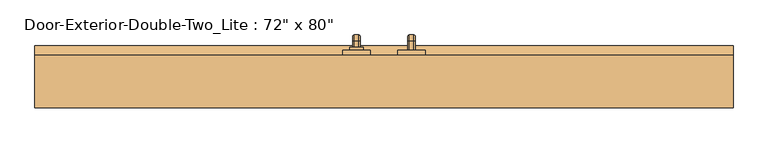
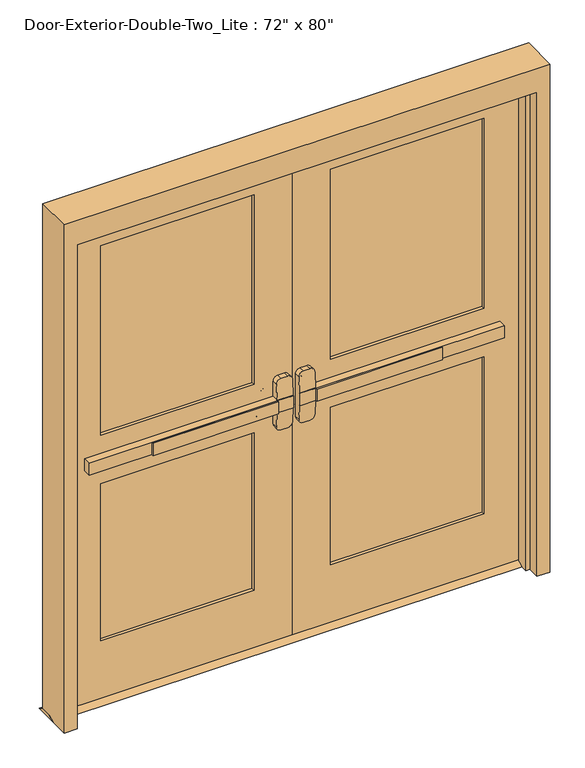
"""IFC4 building model written with IfcOpenShell, lengths in millimetres: door geometry."""

from ifc_helpers import new_model, si_unit, point, frame, frame_2d, origin, place, context, project, spatial, polyline, circle_curve, ellipse_curve, trimmed, segment, composite_curve, outline, extrude, faceted_brep, source, transform, mapped, element, save
from ifc_brep_helpers import plane_surface, cylinder_surface, revolved_surface, advanced_brep


def door_80c43283(model_context):
    return source(origin(), model_context, "Body", "SolidModel", [
        extrude(outline(polyline([(-575.7333333, 0.0), (-575.7333333, 6.35), (-76.2, 6.35), (-76.2, 0.0), (-575.7333333, 0.0)])), frame((0.0, 0.0, 990.6), z_axis=(0.0, 0.0, 1.0), x_axis=(1.0, 0.0, 0.0)), (0.0, 0.0, 1.0), 50.8),
        advanced_brep(
        [(-12.7, 6.35, 1041.4), (-76.2, 6.35, 1041.4), (-825.5, 6.35, 1041.4), (-825.5, 6.35, 990.6), (-76.2, 6.35, 990.6), (-12.7, 6.35, 990.6), (-825.5, 38.1, 1041.4), (-76.2, 38.1, 1041.4), (-76.2, 38.1, 1104.9), (-57.15, 38.1, 1123.95), (-31.75, 38.1, 1123.95), (-12.7, 38.1, 1104.9), (-12.7, 38.1, 927.1), (-31.75, 38.1, 908.05), (-57.15, 38.1, 908.05), (-76.2, 38.1, 927.1), (-76.2, 38.1, 990.6), (-825.5, 38.1, 990.6), (-12.7, 9.5252467, 1041.4), (-76.2, 9.5252467, 1041.4), (-12.7, 9.5252467, 990.6), (-12.7, 14.5354269, 927.1), (-12.7, 14.5354269, 1104.9), (-76.2, 9.5252467, 990.6), (-76.2, 14.5354269, 1104.9), (-76.2, 14.5354269, 927.1), (-57.15, 16.038481, 1123.95), (-31.75, 16.038481, 1123.95), (-31.75, 16.038481, 908.05), (-57.15, 16.038481, 908.05)],
        [
            (0, 1),
            (1, 2),
            (2, 3),
            (3, 4),
            (4, 5),
            (5, 0),
            (6, 7),
            (7, 8),
            (8, 9, circle_curve(frame((-57.15, 38.1, 1104.9), z_axis=(0.0, 1.0, 0.0), x_axis=(-1.0, 0.0, 0.0)), 19.05)),
            (9, 10),
            (10, 11, circle_curve(frame((-31.75, 38.1, 1104.9), z_axis=(0.0, 1.0, 0.0), x_axis=(-1.0, 0.0, 0.0)), 19.05)),
            (11, 12),
            (12, 13, circle_curve(frame((-31.75, 38.1, 927.1), z_axis=(0.0, 1.0, 0.0), x_axis=(-1.0, 0.0, 0.0)), 19.05)),
            (13, 14),
            (14, 15, circle_curve(frame((-57.15, 38.1, 927.1), z_axis=(0.0, 1.0, 0.0), x_axis=(-1.0, 0.0, 0.0)), 19.05)),
            (15, 16),
            (16, 17),
            (17, 6),
            (0, 18),
            (18, 19),
            (19, 7),
            (6, 2),
            (5, 20),
            (20, 21),
            (21, 12),
            (11, 22),
            (22, 18),
            (16, 23),
            (23, 20),
            (3, 17),
            (19, 24),
            (24, 8),
            (15, 25),
            (25, 23),
            (9, 26),
            (26, 27),
            (27, 10),
            (13, 28),
            (28, 29),
            (29, 14),
            (29, 25, ellipse_curve(frame((-57.15, 14.5354269, 927.1), z_axis=(0.0, 0.9969018152893365, 0.07865602756830282), x_axis=(0.0, -0.07865602756830208, 0.9969018152893365)), 19.1092038, 19.05)),
            (24, 26, ellipse_curve(frame((-57.15, 14.5354269, 1104.9), z_axis=(0.0, 0.9969018152893376, -0.07865602756828934), x_axis=(0.0, -0.078656027568288, -0.9969018152893377)), 19.1092038, 19.05)),
            (27, 22, ellipse_curve(frame((-31.75, 14.5354269, 1104.9), z_axis=(0.0, 0.9969018152893376, -0.07865602756828934), x_axis=(0.0, -0.078656027568288, -0.9969018152893377)), 19.1092038, 19.05)),
            (21, 28, ellipse_curve(frame((-31.75, 14.5354269, 927.1), z_axis=(0.0, 0.9969018152893365, 0.07865602756830282), x_axis=(0.0, -0.07865602756830208, 0.9969018152893365)), 19.1092038, 19.05)),
        ],
        [
            plane_surface(frame((-12.7, 6.35, 1041.4), z_axis=(0.0, -1.0, 0.0), x_axis=(1.0, 0.0, 0.0))),
            plane_surface(frame((-12.7, 38.1, 1041.4), z_axis=(0.0, 1.0, 0.0), x_axis=(-1.0, 0.0, 0.0))),
            plane_surface(frame((-825.5, 6.35, 1041.4), z_axis=(0.0, 0.0, 1.0), x_axis=(0.0, 1.0, 0.0))),
            plane_surface(frame((-12.7, 6.35, 1041.4), z_axis=(1.0, 0.0, 0.0), x_axis=(0.0, 1.0, 0.0))),
            plane_surface(frame((-12.7, 6.35, 990.6), z_axis=(0.0, 0.0, -1.0), x_axis=(0.0, 1.0, 0.0))),
            plane_surface(frame((-825.5, 6.35, 990.6), z_axis=(-1.0, 0.0, 0.0), x_axis=(0.0, 1.0, 0.0))),
            plane_surface(frame((-76.2, 9.5252467, 927.1), z_axis=(-1.0, 0.0, 0.0), x_axis=(0.0, 1.0, 0.0))),
            plane_surface(frame((-57.15, 9.5252467, 1123.95), z_axis=(0.0, 0.0, 1.0), x_axis=(0.0, 1.0, 0.0))),
            plane_surface(frame((-31.75, 9.5252467, 908.05), z_axis=(0.0, 0.0, -1.0), x_axis=(0.0, 1.0, 0.0))),
            cylinder_surface(frame((-57.15, 38.1, 927.1), z_axis=(0.0, -1.0, 0.0), x_axis=(-1.0, 0.0, 0.0)), 19.05),
            cylinder_surface(frame((-57.15, 38.1, 1104.9), z_axis=(0.0, -1.0, 0.0), x_axis=(-1.0, 0.0, 0.0)), 19.05),
            cylinder_surface(frame((-31.75, 38.1, 1104.9), z_axis=(0.0, -1.0, 0.0), x_axis=(-1.0, 0.0, 0.0)), 19.05),
            cylinder_surface(frame((-31.75, 38.1, 927.1), z_axis=(0.0, -1.0, 0.0), x_axis=(-1.0, 0.0, 0.0)), 19.05),
            plane_surface(frame((-76.2, 9.5252467, 1041.4), z_axis=(0.0, -0.9969018152893376, 0.07865602756828934), x_axis=(1.0, 0.0, 0.0))),
            plane_surface(frame((-76.2, 16.038481, 908.05), z_axis=(0.0, -0.9969018152893365, -0.07865602756830282), x_axis=(1.0, 0.0, 0.0))),
        ],
        [
            (0, [[1, 2, 3, 4, 5, 6]]),
            (1, [[7, 8, 9, 10, 11, 12, 13, 14, 15, 16, 17, 18]]),
            (2, [[-2, -1, 19, 20, 21, -7, 22]]),
            (3, [[23, 24, 25, -12, 26, 27, -19, -6]]),
            (4, [[-17, 28, 29, -23, -5, -4, 30]]),
            (5, [[-22, -18, -30, -3]]),
            (6, [[-21, 31, 32, -8]]),
            (6, [[33, 34, -28, -16]]),
            (7, [[35, 36, 37, -10]]),
            (8, [[38, 39, 40, -14]]),
            (9, [[-40, 41, -33, -15]]),
            (10, [[-32, 42, -35, -9]]),
            (11, [[-37, 43, -26, -11]]),
            (12, [[-25, 44, -38, -13]]),
            (13, [[-27, -43, -36, -42, -31, -20]]),
            (14, [[-29, -34, -41, -39, -44, -24]]),
        ],
    ),
        extrude(outline(polyline([(82.55, 12.7), (107.95, 0.0), (12.7, 0.0), (38.1, 12.7), (82.55, 12.7)])), frame((-965.2, 0.0, 0.0), z_axis=(1.0, 0.0, 0.0), x_axis=(0.0, 1.0, 0.0)), (0.0, 0.0, 1.0), 1930.4),
        extrude(outline(polyline([(575.7333333, 0.0), (76.2, 0.0), (76.2, 6.35), (575.7333333, 6.35), (575.7333333, 0.0)])), frame((0.0, 0.0, 990.6), z_axis=(0.0, 0.0, 1.0), x_axis=(1.0, 0.0, 0.0)), (0.0, 0.0, 1.0), 50.8),
        advanced_brep(
        [(12.7, 6.35, 1041.4), (12.7, 6.35, 990.6), (76.2, 6.35, 990.6), (825.5, 6.35, 990.6), (825.5, 6.35, 1041.4), (76.2, 6.35, 1041.4), (825.5, 38.1, 1041.4), (825.5, 38.1, 990.6), (76.2, 38.1, 990.6), (76.2, 38.1, 927.1), (57.15, 38.1, 908.05), (31.75, 38.1, 908.05), (12.7, 38.1, 927.1), (12.7, 38.1, 1104.9), (31.75, 38.1, 1123.95), (57.15, 38.1, 1123.95), (76.2, 38.1, 1104.9), (76.2, 38.1, 1041.4), (76.2, 9.5252467, 1041.4), (12.7, 9.5252467, 1041.4), (12.7, 14.5354269, 1104.9), (12.7, 14.5354269, 927.1), (12.7, 9.5252467, 990.6), (76.2, 9.5252467, 990.6), (76.2, 14.5354269, 927.1), (76.2, 14.5354269, 1104.9), (31.75, 16.038481, 1123.95), (57.15, 16.038481, 1123.95), (57.15, 16.038481, 908.05), (31.75, 16.038481, 908.05)],
        [
            (0, 1),
            (1, 2),
            (2, 3),
            (3, 4),
            (4, 5),
            (5, 0),
            (6, 7),
            (7, 8),
            (8, 9),
            (9, 10, circle_curve(frame((57.15, 38.1, 927.1), z_axis=(0.0, 1.0, 0.0), x_axis=(1.0, 0.0, 0.0)), 19.05)),
            (10, 11),
            (11, 12, circle_curve(frame((31.75, 38.1, 927.1), z_axis=(0.0, 1.0, 0.0), x_axis=(1.0, 0.0, 0.0)), 19.05)),
            (12, 13),
            (13, 14, circle_curve(frame((31.75, 38.1, 1104.9), z_axis=(0.0, 1.0, 0.0), x_axis=(1.0, 0.0, 0.0)), 19.05)),
            (14, 15),
            (15, 16, circle_curve(frame((57.15, 38.1, 1104.9), z_axis=(0.0, 1.0, 0.0), x_axis=(1.0, 0.0, 0.0)), 19.05)),
            (16, 17),
            (17, 6),
            (4, 6),
            (17, 18),
            (18, 19),
            (19, 0),
            (19, 20),
            (20, 13),
            (12, 21),
            (21, 22),
            (22, 1),
            (7, 3),
            (22, 23),
            (23, 8),
            (23, 24),
            (24, 9),
            (16, 25),
            (25, 18),
            (14, 26),
            (26, 27),
            (27, 15),
            (10, 28),
            (28, 29),
            (29, 11),
            (24, 28, ellipse_curve(frame((57.15, 14.5354269, 927.1), z_axis=(0.0, 0.9969018152893365, 0.07865602756830282), x_axis=(0.0, -0.07865602756830208, 0.9969018152893365)), 19.1092038, 19.05)),
            (27, 25, ellipse_curve(frame((57.15, 14.5354269, 1104.9), z_axis=(0.0, 0.9969018152893376, -0.07865602756828934), x_axis=(0.0, -0.078656027568288, -0.9969018152893377)), 19.1092038, 19.05)),
            (20, 26, ellipse_curve(frame((31.75, 14.5354269, 1104.9), z_axis=(0.0, 0.9969018152893376, -0.07865602756828934), x_axis=(0.0, -0.078656027568288, -0.9969018152893377)), 19.1092038, 19.05)),
            (29, 21, ellipse_curve(frame((31.75, 14.5354269, 927.1), z_axis=(0.0, 0.9969018152893365, 0.07865602756830282), x_axis=(0.0, -0.07865602756830208, 0.9969018152893365)), 19.1092038, 19.05)),
        ],
        [
            plane_surface(frame((12.7, 6.35, 1041.4), z_axis=(0.0, -1.0, 0.0), x_axis=(-1.0, 0.0, 0.0))),
            plane_surface(frame((12.7, 38.1, 1041.4), z_axis=(0.0, 1.0, 0.0), x_axis=(1.0, 0.0, 0.0))),
            plane_surface(frame((825.5, 6.35, 1041.4), z_axis=(0.0, 0.0, 1.0), x_axis=(0.0, 1.0, 0.0))),
            plane_surface(frame((12.7, 6.35, 1041.4), z_axis=(-1.0, 0.0, 0.0), x_axis=(0.0, 1.0, 0.0))),
            plane_surface(frame((12.7, 6.35, 990.6), z_axis=(0.0, 0.0, -1.0), x_axis=(0.0, 1.0, 0.0))),
            plane_surface(frame((825.5, 6.35, 990.6), z_axis=(1.0, 0.0, 0.0), x_axis=(0.0, 1.0, 0.0))),
            plane_surface(frame((76.2, 9.5252467, 927.1), z_axis=(1.0, 0.0, 0.0), x_axis=(0.0, 1.0, 0.0))),
            plane_surface(frame((57.15, 9.5252467, 1123.95), z_axis=(0.0, 0.0, 1.0), x_axis=(0.0, 1.0, 0.0))),
            plane_surface(frame((31.75, 9.5252467, 908.05), z_axis=(0.0, 0.0, -1.0), x_axis=(0.0, 1.0, 0.0))),
            cylinder_surface(frame((57.15, 38.1, 927.1), z_axis=(0.0, -1.0, 0.0), x_axis=(1.0, 0.0, 0.0)), 19.05),
            cylinder_surface(frame((57.15, 38.1, 1104.9), z_axis=(0.0, -1.0, 0.0), x_axis=(1.0, 0.0, 0.0)), 19.05),
            cylinder_surface(frame((31.75, 38.1, 1104.9), z_axis=(0.0, -1.0, 0.0), x_axis=(1.0, 0.0, 0.0)), 19.05),
            cylinder_surface(frame((31.75, 38.1, 927.1), z_axis=(0.0, -1.0, 0.0), x_axis=(1.0, 0.0, 0.0)), 19.05),
            plane_surface(frame((76.2, 9.5252467, 1041.4), z_axis=(0.0, -0.9969018152893376, 0.07865602756828934), x_axis=(-1.0, 0.0, 0.0))),
            plane_surface(frame((76.2, 16.038481, 908.05), z_axis=(0.0, -0.9969018152893365, -0.07865602756830282), x_axis=(-1.0, 0.0, 0.0))),
        ],
        [
            (0, [[1, 2, 3, 4, 5, 6]]),
            (1, [[7, 8, 9, 10, 11, 12, 13, 14, 15, 16, 17, 18]]),
            (2, [[19, -18, 20, 21, 22, -6, -5]]),
            (3, [[-1, -22, 23, 24, -13, 25, 26, 27]]),
            (4, [[28, -3, -2, -27, 29, 30, -8]]),
            (5, [[-4, -28, -7, -19]]),
            (6, [[-9, -30, 31, 32]]),
            (6, [[-17, 33, 34, -20]]),
            (7, [[-15, 35, 36, 37]]),
            (8, [[-11, 38, 39, 40]]),
            (9, [[-10, -32, 41, -38]]),
            (10, [[-16, -37, 42, -33]]),
            (11, [[-14, -24, 43, -35]]),
            (12, [[-12, -40, 44, -25]]),
            (13, [[-21, -34, -42, -36, -43, -23]]),
            (14, [[-26, -44, -39, -41, -31, -29]]),
        ],
    ),
        advanced_brep(
        [(66.2, 95.25, 1017.190625), (66.2, 95.25, 1014.809375), (69.771875, 95.25, 1011.2375), (82.6284594, 95.25, 1011.2375), (86.2, 95.25, 1014.8090406), (86.2, 95.25, 1017.190625), (82.628125, 95.25, 1020.7625), (69.771875, 95.25, 1020.7625), (66.2, 95.25, 887.809375), (69.771875, 95.25, 884.2375), (82.628125, 95.25, 884.2375), (86.2, 95.25, 887.809375), (86.2, 95.25, 890.1909594), (82.6284594, 95.25, 893.7625), (69.771875, 95.25, 893.7625), (66.2, 95.25, 890.190625), (66.2, 120.65, 1017.190625), (66.2, 134.540625, 1003.3), (66.2, 134.540625, 901.7), (66.2, 120.65, 887.809375), (66.2, 120.65, 890.190625), (66.2, 132.159375, 901.7), (66.2, 132.159375, 1003.3), (66.2, 120.65, 1014.809375), (69.771875, 120.65, 1011.2375), (82.6284594, 120.65, 1011.2375), (86.2, 120.65, 1014.8090406), (86.2, 132.1590406, 1003.3), (86.2, 132.1590406, 901.7), (86.2, 120.65, 890.1909594), (86.2, 120.65, 887.809375), (86.2, 134.540625, 901.7), (86.2, 134.540625, 1003.3), (86.2, 120.65, 1017.190625), (82.628125, 120.65, 1020.7625), (69.771875, 120.65, 1020.7625), (69.771875, 128.5875, 1003.3), (82.6284594, 128.5875, 1003.3), (82.628125, 138.1125, 1003.3), (69.771875, 138.1125, 1003.3), (69.771875, 128.5875, 901.7), (82.6284594, 128.5875, 901.7), (82.628125, 138.1125, 901.7), (69.771875, 138.1125, 901.7), (69.771875, 120.65, 893.7625), (82.6284594, 120.65, 893.7625), (82.628125, 120.65, 884.2375), (69.771875, 120.65, 884.2375)],
        [
            (0, 1),
            (1, 2, circle_curve(frame((69.771875, 95.25, 1014.809375), z_axis=(0.0, -1.0, 0.0), x_axis=(0.0, 0.0, 1.0)), 3.571875)),
            (2, 3),
            (3, 4, circle_curve(frame((82.6284594, 95.25, 1014.8090406), z_axis=(0.0, -1.0, 0.0), x_axis=(0.0, 0.0, 1.0)), 3.5715406)),
            (4, 5),
            (5, 6, circle_curve(frame((82.628125, 95.25, 1017.190625), z_axis=(0.0, -1.0, 0.0), x_axis=(0.0, 0.0, 1.0)), 3.571875)),
            (6, 7),
            (7, 0, circle_curve(frame((69.771875, 95.25, 1017.190625), z_axis=(0.0, -1.0, 0.0), x_axis=(0.0, 0.0, 1.0)), 3.571875)),
            (8, 9, circle_curve(frame((69.771875, 95.25, 887.809375), z_axis=(0.0, -1.0, 0.0), x_axis=(0.0, 0.0, -1.0)), 3.571875)),
            (9, 10),
            (10, 11, circle_curve(frame((82.628125, 95.25, 887.809375), z_axis=(0.0, -1.0, 0.0), x_axis=(0.0, 0.0, -1.0)), 3.571875)),
            (11, 12),
            (12, 13, circle_curve(frame((82.6284594, 95.25, 890.1909594), z_axis=(0.0, -1.0, 0.0), x_axis=(0.0, 0.0, -1.0)), 3.5715406)),
            (13, 14),
            (14, 15, circle_curve(frame((69.771875, 95.25, 890.190625), z_axis=(0.0, -1.0, 0.0), x_axis=(0.0, 0.0, -1.0)), 3.571875)),
            (15, 8),
            (0, 16),
            (16, 17, circle_curve(frame((66.2, 120.65, 1003.3), z_axis=(-1.0, 0.0, 0.0), x_axis=(0.0, 0.0, 1.0)), 13.890625)),
            (17, 18),
            (18, 19, circle_curve(frame((66.2, 120.65, 901.7), z_axis=(-1.0, 0.0, 0.0), x_axis=(0.0, 1.0, 0.0)), 13.890625)),
            (19, 8),
            (15, 20),
            (20, 21, circle_curve(frame((66.2, 120.65, 901.7), z_axis=(1.0, 0.0, 0.0), x_axis=(0.0, 1.0, 0.0)), 11.509375)),
            (21, 22),
            (22, 23, circle_curve(frame((66.2, 120.65, 1003.3), z_axis=(1.0, 0.0, 0.0), x_axis=(0.0, 0.0, 1.0)), 11.509375)),
            (23, 1),
            (23, 24, circle_curve(frame((69.771875, 120.65, 1014.809375), z_axis=(0.0, -1.0, 0.0), x_axis=(0.0, 0.0, 1.0)), 3.571875)),
            (24, 2),
            (24, 25),
            (25, 3),
            (25, 26, circle_curve(frame((82.6284594, 120.65, 1014.8090406), z_axis=(0.0, -1.0, 0.0), x_axis=(0.0, 0.0, 1.0)), 3.5715406)),
            (26, 4),
            (26, 27, circle_curve(frame((86.2, 120.65, 1003.3), z_axis=(-1.0, 0.0, 0.0), x_axis=(0.0, 0.0, 1.0)), 11.5090406)),
            (27, 28),
            (28, 29, circle_curve(frame((86.2, 120.65, 901.7), z_axis=(-1.0, 0.0, 0.0), x_axis=(0.0, 1.0, 0.0)), 11.5090406)),
            (29, 12),
            (11, 30),
            (30, 31, circle_curve(frame((86.2, 120.65, 901.7), z_axis=(1.0, 0.0, 0.0), x_axis=(0.0, 1.0, 0.0)), 13.890625)),
            (31, 32),
            (32, 33, circle_curve(frame((86.2, 120.65, 1003.3), z_axis=(1.0, 0.0, 0.0), x_axis=(0.0, 0.0, 1.0)), 13.890625)),
            (33, 5),
            (33, 34, circle_curve(frame((82.628125, 120.65, 1017.190625), z_axis=(0.0, -1.0, 0.0), x_axis=(0.0, 0.0, 1.0)), 3.571875)),
            (34, 6),
            (34, 35),
            (35, 7),
            (35, 16, circle_curve(frame((69.771875, 120.65, 1017.190625), z_axis=(0.0, -1.0, 0.0), x_axis=(0.0, 0.0, 1.0)), 3.571875)),
            (36, 24, circle_curve(frame((69.771875, 120.65, 1003.3), z_axis=(1.0, 0.0, 0.0), x_axis=(0.0, 0.0, 1.0)), 7.9375)),
            (22, 36, circle_curve(frame((69.771875, 132.159375, 1003.3), z_axis=(0.0, 0.0, 1.0), x_axis=(0.0, 1.0, 0.0)), 3.571875)),
            (37, 25, circle_curve(frame((82.6284594, 120.65, 1003.3), z_axis=(1.0, 0.0, 0.0), x_axis=(0.0, 0.0, 1.0)), 7.9375)),
            (36, 37),
            (37, 27, circle_curve(frame((82.6284594, 132.1590406, 1003.3), z_axis=(0.0, 0.0, 1.0), x_axis=(0.0, 1.0, 0.0)), 3.5715406)),
            (38, 34, circle_curve(frame((82.628125, 120.65, 1003.3), z_axis=(1.0, 0.0, 0.0), x_axis=(0.0, 0.0, 1.0)), 17.4625)),
            (32, 38, circle_curve(frame((82.628125, 134.540625, 1003.3), z_axis=(0.0, 0.0, 1.0), x_axis=(0.0, 1.0, 0.0)), 3.571875)),
            (39, 35, circle_curve(frame((69.771875, 120.65, 1003.3), z_axis=(1.0, 0.0, 0.0), x_axis=(0.0, 0.0, 1.0)), 17.4625)),
            (38, 39),
            (39, 17, circle_curve(frame((69.771875, 134.540625, 1003.3), z_axis=(0.0, 0.0, 1.0), x_axis=(0.0, 1.0, 0.0)), 3.571875)),
            (21, 40, circle_curve(frame((69.771875, 132.159375, 901.7), z_axis=(0.0, 0.0, 1.0), x_axis=(0.0, 1.0, 0.0)), 3.571875)),
            (40, 36),
            (40, 41),
            (41, 37),
            (41, 28, circle_curve(frame((82.6284594, 132.1590406, 901.7), z_axis=(0.0, 0.0, 1.0), x_axis=(0.0, 1.0, 0.0)), 3.5715406)),
            (31, 42, circle_curve(frame((82.628125, 134.540625, 901.7), z_axis=(0.0, 0.0, 1.0), x_axis=(0.0, 1.0, 0.0)), 3.571875)),
            (42, 38),
            (42, 43),
            (43, 39),
            (43, 18, circle_curve(frame((69.771875, 134.540625, 901.7), z_axis=(0.0, 0.0, 1.0), x_axis=(0.0, 1.0, 0.0)), 3.571875)),
            (44, 40, circle_curve(frame((69.771875, 120.65, 901.7), z_axis=(1.0, 0.0, 0.0), x_axis=(0.0, 1.0, 0.0)), 7.9375)),
            (20, 44, circle_curve(frame((69.771875, 120.65, 890.190625), z_axis=(0.0, 1.0, 0.0), x_axis=(0.0, 0.0, -1.0)), 3.571875)),
            (45, 41, circle_curve(frame((82.6284594, 120.65, 901.7), z_axis=(1.0, 0.0, 0.0), x_axis=(0.0, 1.0, 0.0)), 7.9375)),
            (44, 45),
            (45, 29, circle_curve(frame((82.6284594, 120.65, 890.1909594), z_axis=(0.0, 1.0, 0.0), x_axis=(0.0, 0.0, -1.0)), 3.5715406)),
            (46, 42, circle_curve(frame((82.628125, 120.65, 901.7), z_axis=(1.0, 0.0, 0.0), x_axis=(0.0, 1.0, 0.0)), 17.4625)),
            (30, 46, circle_curve(frame((82.628125, 120.65, 887.809375), z_axis=(0.0, 1.0, 0.0), x_axis=(0.0, 0.0, -1.0)), 3.571875)),
            (47, 43, circle_curve(frame((69.771875, 120.65, 901.7), z_axis=(1.0, 0.0, 0.0), x_axis=(0.0, 1.0, 0.0)), 17.4625)),
            (46, 47),
            (47, 19, circle_curve(frame((69.771875, 120.65, 887.809375), z_axis=(0.0, 1.0, 0.0), x_axis=(0.0, 0.0, -1.0)), 3.571875)),
            (14, 44),
            (13, 45),
            (10, 46),
            (9, 47),
        ],
        [
            plane_surface(frame((76.2, 95.25, 1016.0), z_axis=(0.0, -1.0, 0.0), x_axis=(1.0, 0.0, 0.0))),
            plane_surface(frame((76.2, 95.25, 889.0), z_axis=(0.0, -1.0, 0.0), x_axis=(1.0, 0.0, 0.0))),
            plane_surface(frame((66.2, 95.25, 1017.190625), z_axis=(-1.0, 0.0, 0.0), x_axis=(0.0, 1.0, 0.0))),
            cylinder_surface(frame((69.771875, 95.25, 1014.809375), z_axis=(0.0, -1.0, 0.0), x_axis=(0.0, 0.0, 1.0)), 3.571875),
            plane_surface(frame((69.771875, 95.25, 1011.2375), z_axis=(0.0, 0.0, -1.0), x_axis=(0.0, 1.0, 0.0))),
            cylinder_surface(frame((82.6284594, 95.25, 1014.8090406), z_axis=(0.0, -1.0, 0.0), x_axis=(0.0, 0.0, 1.0)), 3.5715406),
            plane_surface(frame((86.2, 95.25, 1014.8090406), z_axis=(1.0, 0.0, 0.0), x_axis=(0.0, 1.0, 0.0))),
            cylinder_surface(frame((82.628125, 95.25, 1017.190625), z_axis=(0.0, -1.0, 0.0), x_axis=(0.0, 0.0, 1.0)), 3.571875),
            plane_surface(frame((82.628125, 95.25, 1020.7625), z_axis=(0.0, 0.0, 1.0), x_axis=(0.0, 1.0, 0.0))),
            cylinder_surface(frame((69.771875, 95.25, 1017.190625), z_axis=(0.0, -1.0, 0.0), x_axis=(0.0, 0.0, 1.0)), 3.571875),
            revolved_surface(trimmed(ellipse_curve(frame((69.771875, 120.65, 1014.809375), z_axis=(0.0, -1.0, 0.0), x_axis=(0.0, 0.0, 1.0)), 3.571875, 3.571875), [point((66.2, 120.65, 1014.809375))], [point((69.771875, 120.65, 1011.2375))], True, "CARTESIAN"), (76.2, 120.65, 1003.3), (-1.0, 0.0, 0.0)),
            revolved_surface(polyline([(69.771875, 120.65, 1011.2375), (82.6284594, 120.65, 1011.2375)]), (76.2, 120.65, 1003.3), (-1.0, 0.0, 0.0)),
            revolved_surface(trimmed(ellipse_curve(frame((82.6284594, 120.65, 1014.8090406), z_axis=(0.0, -1.0, 0.0), x_axis=(0.0, 0.0, 1.0)), 3.5715406, 3.5715406), [point((82.6284594, 120.65, 1011.2375))], [point((86.2, 120.65, 1014.8090406))], True, "CARTESIAN"), (76.2, 120.65, 1003.3), (-1.0, 0.0, 0.0)),
            revolved_surface(trimmed(ellipse_curve(frame((82.628125, 120.65, 1017.190625), z_axis=(0.0, -1.0, 0.0), x_axis=(0.0, 0.0, 1.0)), 3.571875, 3.571875), [point((86.2, 120.65, 1017.190625))], [point((82.628125, 120.65, 1020.7625))], True, "CARTESIAN"), (76.2, 120.65, 1003.3), (-1.0, 0.0, 0.0)),
            cylinder_surface(frame((76.2, 120.65, 1003.3), z_axis=(-1.0, 0.0, 0.0), x_axis=(0.0, 0.0, 1.0)), 17.4625),
            revolved_surface(trimmed(ellipse_curve(frame((69.771875, 120.65, 1017.190625), z_axis=(0.0, -1.0, 0.0), x_axis=(0.0, 0.0, 1.0)), 3.571875, 3.571875), [point((69.771875, 120.65, 1020.7625))], [point((66.2, 120.65, 1017.190625))], True, "CARTESIAN"), (76.2, 120.65, 1003.3), (-1.0, 0.0, 0.0)),
            cylinder_surface(frame((69.771875, 132.159375, 1003.3), z_axis=(0.0, 0.0, 1.0), x_axis=(0.0, 1.0, 0.0)), 3.571875),
            plane_surface(frame((69.771875, 128.5875, 1003.3), z_axis=(0.0, -1.0, 0.0), x_axis=(0.0, 0.0, -1.0))),
            cylinder_surface(frame((82.6284594, 132.1590406, 1003.3), z_axis=(0.0, 0.0, 1.0), x_axis=(0.0, 1.0, 0.0)), 3.5715406),
            cylinder_surface(frame((82.628125, 134.540625, 1003.3), z_axis=(0.0, 0.0, 1.0), x_axis=(0.0, 1.0, 0.0)), 3.571875),
            plane_surface(frame((82.628125, 138.1125, 1003.3), z_axis=(0.0, 1.0, 0.0), x_axis=(0.0, 0.0, -1.0))),
            cylinder_surface(frame((69.771875, 134.540625, 1003.3), z_axis=(0.0, 0.0, 1.0), x_axis=(0.0, 1.0, 0.0)), 3.571875),
            revolved_surface(trimmed(ellipse_curve(frame((69.771875, 132.159375, 901.7), z_axis=(0.0, 0.0, 1.0), x_axis=(0.0, 1.0, 0.0)), 3.571875, 3.571875), [point((66.2, 132.159375, 901.7))], [point((69.771875, 128.5875, 901.7))], True, "CARTESIAN"), (76.2, 120.65, 901.7), (-1.0, 0.0, 0.0)),
            revolved_surface(polyline([(69.771875, 128.5875, 901.7), (82.6284594, 128.5875, 901.7)]), (76.2, 120.65, 901.7), (-1.0, 0.0, 0.0)),
            revolved_surface(trimmed(ellipse_curve(frame((82.6284594, 132.1590406, 901.7), z_axis=(0.0, 0.0, 1.0), x_axis=(0.0, 1.0, 0.0)), 3.5715406, 3.5715406), [point((82.6284594, 128.5875, 901.7))], [point((86.2, 132.1590406, 901.7))], True, "CARTESIAN"), (76.2, 120.65, 901.7), (-1.0, 0.0, 0.0)),
            revolved_surface(trimmed(ellipse_curve(frame((82.628125, 134.540625, 901.7), z_axis=(0.0, 0.0, 1.0), x_axis=(0.0, 1.0, 0.0)), 3.571875, 3.571875), [point((86.2, 134.540625, 901.7))], [point((82.628125, 138.1125, 901.7))], True, "CARTESIAN"), (76.2, 120.65, 901.7), (-1.0, 0.0, 0.0)),
            cylinder_surface(frame((76.2, 120.65, 901.7), z_axis=(-1.0, 0.0, 0.0), x_axis=(0.0, 1.0, 0.0)), 17.4625),
            revolved_surface(trimmed(ellipse_curve(frame((69.771875, 134.540625, 901.7), z_axis=(0.0, 0.0, 1.0), x_axis=(0.0, 1.0, 0.0)), 3.571875, 3.571875), [point((69.771875, 138.1125, 901.7))], [point((66.2, 134.540625, 901.7))], True, "CARTESIAN"), (76.2, 120.65, 901.7), (-1.0, 0.0, 0.0)),
            cylinder_surface(frame((69.771875, 120.65, 890.190625), z_axis=(0.0, 1.0, 0.0), x_axis=(0.0, 0.0, -1.0)), 3.571875),
            plane_surface(frame((69.771875, 120.65, 893.7625), z_axis=(0.0, 0.0, 1.0), x_axis=(0.0, -1.0, 0.0))),
            cylinder_surface(frame((82.6284594, 120.65, 890.1909594), z_axis=(0.0, 1.0, 0.0), x_axis=(0.0, 0.0, -1.0)), 3.5715406),
            cylinder_surface(frame((82.628125, 120.65, 887.809375), z_axis=(0.0, 1.0, 0.0), x_axis=(0.0, 0.0, -1.0)), 3.571875),
            plane_surface(frame((82.628125, 120.65, 884.2375), z_axis=(0.0, 0.0, -1.0), x_axis=(0.0, -1.0, 0.0))),
            cylinder_surface(frame((69.771875, 120.65, 887.809375), z_axis=(0.0, 1.0, 0.0), x_axis=(0.0, 0.0, -1.0)), 3.571875),
        ],
        [
            (0, [[1, 2, 3, 4, 5, 6, 7, 8]]),
            (1, [[9, 10, 11, 12, 13, 14, 15, 16]]),
            (2, [[-1, 17, 18, 19, 20, 21, -16, 22, 23, 24, 25, 26]]),
            (3, [[-2, -26, 27, 28]]),
            (4, [[-3, -28, 29, 30]]),
            (5, [[-4, -30, 31, 32]]),
            (6, [[-5, -32, 33, 34, 35, 36, -12, 37, 38, 39, 40, 41]]),
            (7, [[-6, -41, 42, 43]]),
            (8, [[-7, -43, 44, 45]]),
            (9, [[-8, -45, 46, -17]]),
            (10, [[47, -27, -25, 48]]),
            (11, [[49, -29, -47, 50]]),
            (12, [[-33, -31, -49, 51]]),
            (13, [[52, -42, -40, 53]]),
            (14, [[54, -44, -52, 55]]),
            (15, [[-18, -46, -54, 56]]),
            (16, [[-48, -24, 57, 58]]),
            (17, [[-50, -58, 59, 60]]),
            (18, [[-51, -60, 61, -34]]),
            (19, [[-53, -39, 62, 63]]),
            (20, [[-55, -63, 64, 65]]),
            (21, [[-56, -65, 66, -19]]),
            (22, [[67, -57, -23, 68]]),
            (23, [[69, -59, -67, 70]]),
            (24, [[-35, -61, -69, 71]]),
            (25, [[72, -62, -38, 73]]),
            (26, [[74, -64, -72, 75]]),
            (27, [[-20, -66, -74, 76]]),
            (28, [[-68, -22, -15, 77]]),
            (29, [[-70, -77, -14, 78]]),
            (30, [[-71, -78, -13, -36]]),
            (31, [[-73, -37, -11, 79]]),
            (32, [[-75, -79, -10, 80]]),
            (33, [[-76, -80, -9, -21]]),
        ],
    ),
        extrude(outline(composite_curve([segment(trimmed(circle_curve(frame_2d((1113.0338574, 76.2)), 89.3016225), [point((1193.8, 114.3))], [point((1193.8, 38.1))], False, "CARTESIAN"), True, "CONTINUOUS"), segment(polyline([(1193.8, 38.1), (838.2, 38.1)]), True, "CONTINUOUS"), segment(trimmed(circle_curve(frame_2d((918.9661426, 76.2)), 89.3016225), [point((838.2, 38.1))], [point((838.2, 114.3))], False, "CARTESIAN"), True, "CONTINUOUS"), segment(polyline([(838.2, 114.3), (1193.8, 114.3)]), True, "CONTINUOUS")], self_intersect=False)), frame((0.0, 82.55, 0.0), z_axis=(0.0, 1.0, 0.0), x_axis=(0.0, 0.0, 1.0)), (0.0, 0.0, 1.0), 12.7),
        advanced_brep(
        [(-86.2, 95.25, 1017.190625), (-86.2, 95.25, 1014.809375), (-82.628125, 95.25, 1011.2375), (-69.7715406, 95.25, 1011.2375), (-66.2, 95.25, 1014.8090406), (-66.2, 95.25, 1017.190625), (-69.771875, 95.25, 1020.7625), (-82.628125, 95.25, 1020.7625), (-86.2, 95.25, 887.809375), (-82.628125, 95.25, 884.2375), (-69.771875, 95.25, 884.2375), (-66.2, 95.25, 887.809375), (-66.2, 95.25, 890.1909594), (-69.7715406, 95.25, 893.7625), (-82.628125, 95.25, 893.7625), (-86.2, 95.25, 890.190625), (-86.2, 120.65, 1017.190625), (-86.2, 134.540625, 1003.3), (-86.2, 134.540625, 901.7), (-86.2, 120.65, 887.809375), (-86.2, 120.65, 890.190625), (-86.2, 132.159375, 901.7), (-86.2, 132.159375, 1003.3), (-86.2, 120.65, 1014.809375), (-82.628125, 120.65, 1011.2375), (-69.7715406, 120.65, 1011.2375), (-66.2, 120.65, 1014.8090406), (-66.2, 132.1590406, 1003.3), (-66.2, 132.1590406, 901.7), (-66.2, 120.65, 890.1909594), (-66.2, 120.65, 887.809375), (-66.2, 134.540625, 901.7), (-66.2, 134.540625, 1003.3), (-66.2, 120.65, 1017.190625), (-69.771875, 120.65, 1020.7625), (-82.628125, 120.65, 1020.7625), (-82.628125, 128.5875, 1003.3), (-69.7715406, 128.5875, 1003.3), (-69.771875, 138.1125, 1003.3), (-82.628125, 138.1125, 1003.3), (-82.628125, 128.5875, 901.7), (-69.7715406, 128.5875, 901.7), (-69.771875, 138.1125, 901.7), (-82.628125, 138.1125, 901.7), (-82.628125, 120.65, 893.7625), (-69.7715406, 120.65, 893.7625), (-69.771875, 120.65, 884.2375), (-82.628125, 120.65, 884.2375)],
        [
            (0, 1),
            (1, 2, circle_curve(frame((-82.628125, 95.25, 1014.809375), z_axis=(0.0, -1.0, 0.0), x_axis=(0.0, 0.0, 1.0)), 3.571875)),
            (2, 3),
            (3, 4, circle_curve(frame((-69.7715406, 95.25, 1014.8090406), z_axis=(0.0, -1.0, 0.0), x_axis=(0.0, 0.0, 1.0)), 3.5715406)),
            (4, 5),
            (5, 6, circle_curve(frame((-69.771875, 95.25, 1017.190625), z_axis=(0.0, -1.0, 0.0), x_axis=(0.0, 0.0, 1.0)), 3.571875)),
            (6, 7),
            (7, 0, circle_curve(frame((-82.628125, 95.25, 1017.190625), z_axis=(0.0, -1.0, 0.0), x_axis=(0.0, 0.0, 1.0)), 3.571875)),
            (8, 9, circle_curve(frame((-82.628125, 95.25, 887.809375), z_axis=(0.0, -1.0, 0.0), x_axis=(0.0, 0.0, -1.0)), 3.571875)),
            (9, 10),
            (10, 11, circle_curve(frame((-69.771875, 95.25, 887.809375), z_axis=(0.0, -1.0, 0.0), x_axis=(0.0, 0.0, -1.0)), 3.571875)),
            (11, 12),
            (12, 13, circle_curve(frame((-69.7715406, 95.25, 890.1909594), z_axis=(0.0, -1.0, 0.0), x_axis=(0.0, 0.0, -1.0)), 3.5715406)),
            (13, 14),
            (14, 15, circle_curve(frame((-82.628125, 95.25, 890.190625), z_axis=(0.0, -1.0, 0.0), x_axis=(0.0, 0.0, -1.0)), 3.571875)),
            (15, 8),
            (0, 16),
            (16, 17, circle_curve(frame((-86.2, 120.65, 1003.3), z_axis=(-1.0, 0.0, 0.0), x_axis=(0.0, 0.0, 1.0)), 13.890625)),
            (17, 18),
            (18, 19, circle_curve(frame((-86.2, 120.65, 901.7), z_axis=(-1.0, 0.0, 0.0), x_axis=(0.0, 1.0, 0.0)), 13.890625)),
            (19, 8),
            (15, 20),
            (20, 21, circle_curve(frame((-86.2, 120.65, 901.7), z_axis=(1.0, 0.0, 0.0), x_axis=(0.0, 1.0, 0.0)), 11.509375)),
            (21, 22),
            (22, 23, circle_curve(frame((-86.2, 120.65, 1003.3), z_axis=(1.0, 0.0, 0.0), x_axis=(0.0, 0.0, 1.0)), 11.509375)),
            (23, 1),
            (23, 24, circle_curve(frame((-82.628125, 120.65, 1014.809375), z_axis=(0.0, -1.0, 0.0), x_axis=(0.0, 0.0, 1.0)), 3.571875)),
            (24, 2),
            (24, 25),
            (25, 3),
            (25, 26, circle_curve(frame((-69.7715406, 120.65, 1014.8090406), z_axis=(0.0, -1.0, 0.0), x_axis=(0.0, 0.0, 1.0)), 3.5715406)),
            (26, 4),
            (26, 27, circle_curve(frame((-66.2, 120.65, 1003.3), z_axis=(-1.0, 0.0, 0.0), x_axis=(0.0, 0.0, 1.0)), 11.5090406)),
            (27, 28),
            (28, 29, circle_curve(frame((-66.2, 120.65, 901.7), z_axis=(-1.0, 0.0, 0.0), x_axis=(0.0, 1.0, 0.0)), 11.5090406)),
            (29, 12),
            (11, 30),
            (30, 31, circle_curve(frame((-66.2, 120.65, 901.7), z_axis=(1.0, 0.0, 0.0), x_axis=(0.0, 1.0, 0.0)), 13.890625)),
            (31, 32),
            (32, 33, circle_curve(frame((-66.2, 120.65, 1003.3), z_axis=(1.0, 0.0, 0.0), x_axis=(0.0, 0.0, 1.0)), 13.890625)),
            (33, 5),
            (33, 34, circle_curve(frame((-69.771875, 120.65, 1017.190625), z_axis=(0.0, -1.0, 0.0), x_axis=(0.0, 0.0, 1.0)), 3.571875)),
            (34, 6),
            (34, 35),
            (35, 7),
            (35, 16, circle_curve(frame((-82.628125, 120.65, 1017.190625), z_axis=(0.0, -1.0, 0.0), x_axis=(0.0, 0.0, 1.0)), 3.571875)),
            (36, 24, circle_curve(frame((-82.628125, 120.65, 1003.3), z_axis=(1.0, 0.0, 0.0), x_axis=(0.0, 0.0, 1.0)), 7.9375)),
            (22, 36, circle_curve(frame((-82.628125, 132.159375, 1003.3), z_axis=(0.0, 0.0, 1.0), x_axis=(0.0, 1.0, 0.0)), 3.571875)),
            (37, 25, circle_curve(frame((-69.7715406, 120.65, 1003.3), z_axis=(1.0, 0.0, 0.0), x_axis=(0.0, 0.0, 1.0)), 7.9375)),
            (36, 37),
            (37, 27, circle_curve(frame((-69.7715406, 132.1590406, 1003.3), z_axis=(0.0, 0.0, 1.0), x_axis=(0.0, 1.0, 0.0)), 3.5715406)),
            (38, 34, circle_curve(frame((-69.771875, 120.65, 1003.3), z_axis=(1.0, 0.0, 0.0), x_axis=(0.0, 0.0, 1.0)), 17.4625)),
            (32, 38, circle_curve(frame((-69.771875, 134.540625, 1003.3), z_axis=(0.0, 0.0, 1.0), x_axis=(0.0, 1.0, 0.0)), 3.571875)),
            (39, 35, circle_curve(frame((-82.628125, 120.65, 1003.3), z_axis=(1.0, 0.0, 0.0), x_axis=(0.0, 0.0, 1.0)), 17.4625)),
            (38, 39),
            (39, 17, circle_curve(frame((-82.628125, 134.540625, 1003.3), z_axis=(0.0, 0.0, 1.0), x_axis=(0.0, 1.0, 0.0)), 3.571875)),
            (21, 40, circle_curve(frame((-82.628125, 132.159375, 901.7), z_axis=(0.0, 0.0, 1.0), x_axis=(0.0, 1.0, 0.0)), 3.571875)),
            (40, 36),
            (40, 41),
            (41, 37),
            (41, 28, circle_curve(frame((-69.7715406, 132.1590406, 901.7), z_axis=(0.0, 0.0, 1.0), x_axis=(0.0, 1.0, 0.0)), 3.5715406)),
            (31, 42, circle_curve(frame((-69.771875, 134.540625, 901.7), z_axis=(0.0, 0.0, 1.0), x_axis=(0.0, 1.0, 0.0)), 3.571875)),
            (42, 38),
            (42, 43),
            (43, 39),
            (43, 18, circle_curve(frame((-82.628125, 134.540625, 901.7), z_axis=(0.0, 0.0, 1.0), x_axis=(0.0, 1.0, 0.0)), 3.571875)),
            (44, 40, circle_curve(frame((-82.628125, 120.65, 901.7), z_axis=(1.0, 0.0, 0.0), x_axis=(0.0, 1.0, 0.0)), 7.9375)),
            (20, 44, circle_curve(frame((-82.628125, 120.65, 890.190625), z_axis=(0.0, 1.0, 0.0), x_axis=(0.0, 0.0, -1.0)), 3.571875)),
            (45, 41, circle_curve(frame((-69.7715406, 120.65, 901.7), z_axis=(1.0, 0.0, 0.0), x_axis=(0.0, 1.0, 0.0)), 7.9375)),
            (44, 45),
            (45, 29, circle_curve(frame((-69.7715406, 120.65, 890.1909594), z_axis=(0.0, 1.0, 0.0), x_axis=(0.0, 0.0, -1.0)), 3.5715406)),
            (46, 42, circle_curve(frame((-69.771875, 120.65, 901.7), z_axis=(1.0, 0.0, 0.0), x_axis=(0.0, 1.0, 0.0)), 17.4625)),
            (30, 46, circle_curve(frame((-69.771875, 120.65, 887.809375), z_axis=(0.0, 1.0, 0.0), x_axis=(0.0, 0.0, -1.0)), 3.571875)),
            (47, 43, circle_curve(frame((-82.628125, 120.65, 901.7), z_axis=(1.0, 0.0, 0.0), x_axis=(0.0, 1.0, 0.0)), 17.4625)),
            (46, 47),
            (47, 19, circle_curve(frame((-82.628125, 120.65, 887.809375), z_axis=(0.0, 1.0, 0.0), x_axis=(0.0, 0.0, -1.0)), 3.571875)),
            (14, 44),
            (13, 45),
            (10, 46),
            (9, 47),
        ],
        [
            plane_surface(frame((-76.2, 95.25, 1016.0), z_axis=(0.0, -1.0, 0.0), x_axis=(1.0, 0.0, 0.0))),
            plane_surface(frame((-76.2, 95.25, 889.0), z_axis=(0.0, -1.0, 0.0), x_axis=(1.0, 0.0, 0.0))),
            plane_surface(frame((-86.2, 95.25, 1017.190625), z_axis=(-1.0, 0.0, 0.0), x_axis=(0.0, 1.0, 0.0))),
            cylinder_surface(frame((-82.628125, 95.25, 1014.809375), z_axis=(0.0, -1.0, 0.0), x_axis=(0.0, 0.0, 1.0)), 3.571875),
            plane_surface(frame((-82.628125, 95.25, 1011.2375), z_axis=(0.0, 0.0, -1.0), x_axis=(0.0, 1.0, 0.0))),
            cylinder_surface(frame((-69.7715406, 95.25, 1014.8090406), z_axis=(0.0, -1.0, 0.0), x_axis=(0.0, 0.0, 1.0)), 3.5715406),
            plane_surface(frame((-66.2, 95.25, 1014.8090406), z_axis=(1.0, 0.0, 0.0), x_axis=(0.0, 1.0, 0.0))),
            cylinder_surface(frame((-69.771875, 95.25, 1017.190625), z_axis=(0.0, -1.0, 0.0), x_axis=(0.0, 0.0, 1.0)), 3.571875),
            plane_surface(frame((-69.771875, 95.25, 1020.7625), z_axis=(0.0, 0.0, 1.0), x_axis=(0.0, 1.0, 0.0))),
            cylinder_surface(frame((-82.628125, 95.25, 1017.190625), z_axis=(0.0, -1.0, 0.0), x_axis=(0.0, 0.0, 1.0)), 3.571875),
            revolved_surface(trimmed(ellipse_curve(frame((-82.628125, 120.65, 1014.809375), z_axis=(0.0, -1.0, 0.0), x_axis=(0.0, 0.0, 1.0)), 3.571875, 3.571875), [point((-86.2, 120.65, 1014.809375))], [point((-82.628125, 120.65, 1011.2375))], True, "CARTESIAN"), (-76.2, 120.65, 1003.3), (-1.0, 0.0, 0.0)),
            revolved_surface(polyline([(-82.628125, 120.65, 1011.2375), (-69.7715406, 120.65, 1011.2375)]), (-76.2, 120.65, 1003.3), (-1.0, 0.0, 0.0)),
            revolved_surface(trimmed(ellipse_curve(frame((-69.7715406, 120.65, 1014.8090406), z_axis=(0.0, -1.0, 0.0), x_axis=(0.0, 0.0, 1.0)), 3.5715406, 3.5715406), [point((-69.7715406, 120.65, 1011.2375))], [point((-66.2, 120.65, 1014.8090406))], True, "CARTESIAN"), (-76.2, 120.65, 1003.3), (-1.0, 0.0, 0.0)),
            revolved_surface(trimmed(ellipse_curve(frame((-69.771875, 120.65, 1017.190625), z_axis=(0.0, -1.0, 0.0), x_axis=(0.0, 0.0, 1.0)), 3.571875, 3.571875), [point((-66.2, 120.65, 1017.190625))], [point((-69.771875, 120.65, 1020.7625))], True, "CARTESIAN"), (-76.2, 120.65, 1003.3), (-1.0, 0.0, 0.0)),
            cylinder_surface(frame((-76.2, 120.65, 1003.3), z_axis=(-1.0, 0.0, 0.0), x_axis=(0.0, 0.0, 1.0)), 17.4625),
            revolved_surface(trimmed(ellipse_curve(frame((-82.628125, 120.65, 1017.190625), z_axis=(0.0, -1.0, 0.0), x_axis=(0.0, 0.0, 1.0)), 3.571875, 3.571875), [point((-82.628125, 120.65, 1020.7625))], [point((-86.2, 120.65, 1017.190625))], True, "CARTESIAN"), (-76.2, 120.65, 1003.3), (-1.0, 0.0, 0.0)),
            cylinder_surface(frame((-82.628125, 132.159375, 1003.3), z_axis=(0.0, 0.0, 1.0), x_axis=(0.0, 1.0, 0.0)), 3.571875),
            plane_surface(frame((-82.628125, 128.5875, 1003.3), z_axis=(0.0, -1.0, 0.0), x_axis=(0.0, 0.0, -1.0))),
            cylinder_surface(frame((-69.7715406, 132.1590406, 1003.3), z_axis=(0.0, 0.0, 1.0), x_axis=(0.0, 1.0, 0.0)), 3.5715406),
            cylinder_surface(frame((-69.771875, 134.540625, 1003.3), z_axis=(0.0, 0.0, 1.0), x_axis=(0.0, 1.0, 0.0)), 3.571875),
            plane_surface(frame((-69.771875, 138.1125, 1003.3), z_axis=(0.0, 1.0, 0.0), x_axis=(0.0, 0.0, -1.0))),
            cylinder_surface(frame((-82.628125, 134.540625, 1003.3), z_axis=(0.0, 0.0, 1.0), x_axis=(0.0, 1.0, 0.0)), 3.571875),
            revolved_surface(trimmed(ellipse_curve(frame((-82.628125, 132.159375, 901.7), z_axis=(0.0, 0.0, 1.0), x_axis=(0.0, 1.0, 0.0)), 3.571875, 3.571875), [point((-86.2, 132.159375, 901.7))], [point((-82.628125, 128.5875, 901.7))], True, "CARTESIAN"), (-76.2, 120.65, 901.7), (-1.0, 0.0, 0.0)),
            revolved_surface(polyline([(-82.628125, 128.5875, 901.7), (-69.7715406, 128.5875, 901.7)]), (-76.2, 120.65, 901.7), (-1.0, 0.0, 0.0)),
            revolved_surface(trimmed(ellipse_curve(frame((-69.7715406, 132.1590406, 901.7), z_axis=(0.0, 0.0, 1.0), x_axis=(0.0, 1.0, 0.0)), 3.5715406, 3.5715406), [point((-69.7715406, 128.5875, 901.7))], [point((-66.2, 132.1590406, 901.7))], True, "CARTESIAN"), (-76.2, 120.65, 901.7), (-1.0, 0.0, 0.0)),
            revolved_surface(trimmed(ellipse_curve(frame((-69.771875, 134.540625, 901.7), z_axis=(0.0, 0.0, 1.0), x_axis=(0.0, 1.0, 0.0)), 3.571875, 3.571875), [point((-66.2, 134.540625, 901.7))], [point((-69.771875, 138.1125, 901.7))], True, "CARTESIAN"), (-76.2, 120.65, 901.7), (-1.0, 0.0, 0.0)),
            cylinder_surface(frame((-76.2, 120.65, 901.7), z_axis=(-1.0, 0.0, 0.0), x_axis=(0.0, 1.0, 0.0)), 17.4625),
            revolved_surface(trimmed(ellipse_curve(frame((-82.628125, 134.540625, 901.7), z_axis=(0.0, 0.0, 1.0), x_axis=(0.0, 1.0, 0.0)), 3.571875, 3.571875), [point((-82.628125, 138.1125, 901.7))], [point((-86.2, 134.540625, 901.7))], True, "CARTESIAN"), (-76.2, 120.65, 901.7), (-1.0, 0.0, 0.0)),
            cylinder_surface(frame((-82.628125, 120.65, 890.190625), z_axis=(0.0, 1.0, 0.0), x_axis=(0.0, 0.0, -1.0)), 3.571875),
            plane_surface(frame((-82.628125, 120.65, 893.7625), z_axis=(0.0, 0.0, 1.0), x_axis=(0.0, -1.0, 0.0))),
            cylinder_surface(frame((-69.7715406, 120.65, 890.1909594), z_axis=(0.0, 1.0, 0.0), x_axis=(0.0, 0.0, -1.0)), 3.5715406),
            cylinder_surface(frame((-69.771875, 120.65, 887.809375), z_axis=(0.0, 1.0, 0.0), x_axis=(0.0, 0.0, -1.0)), 3.571875),
            plane_surface(frame((-69.771875, 120.65, 884.2375), z_axis=(0.0, 0.0, -1.0), x_axis=(0.0, -1.0, 0.0))),
            cylinder_surface(frame((-82.628125, 120.65, 887.809375), z_axis=(0.0, 1.0, 0.0), x_axis=(0.0, 0.0, -1.0)), 3.571875),
        ],
        [
            (0, [[1, 2, 3, 4, 5, 6, 7, 8]]),
            (1, [[9, 10, 11, 12, 13, 14, 15, 16]]),
            (2, [[-1, 17, 18, 19, 20, 21, -16, 22, 23, 24, 25, 26]]),
            (3, [[-2, -26, 27, 28]]),
            (4, [[-3, -28, 29, 30]]),
            (5, [[-4, -30, 31, 32]]),
            (6, [[-5, -32, 33, 34, 35, 36, -12, 37, 38, 39, 40, 41]]),
            (7, [[-6, -41, 42, 43]]),
            (8, [[-7, -43, 44, 45]]),
            (9, [[-8, -45, 46, -17]]),
            (10, [[47, -27, -25, 48]]),
            (11, [[49, -29, -47, 50]]),
            (12, [[-33, -31, -49, 51]]),
            (13, [[52, -42, -40, 53]]),
            (14, [[54, -44, -52, 55]]),
            (15, [[-18, -46, -54, 56]]),
            (16, [[-48, -24, 57, 58]]),
            (17, [[-50, -58, 59, 60]]),
            (18, [[-51, -60, 61, -34]]),
            (19, [[-53, -39, 62, 63]]),
            (20, [[-55, -63, 64, 65]]),
            (21, [[-56, -65, 66, -19]]),
            (22, [[67, -57, -23, 68]]),
            (23, [[69, -59, -67, 70]]),
            (24, [[-35, -61, -69, 71]]),
            (25, [[72, -62, -38, 73]]),
            (26, [[74, -64, -72, 75]]),
            (27, [[-20, -66, -74, 76]]),
            (28, [[-68, -22, -15, 77]]),
            (29, [[-70, -77, -14, 78]]),
            (30, [[-71, -78, -13, -36]]),
            (31, [[-73, -37, -11, 79]]),
            (32, [[-75, -79, -10, 80]]),
            (33, [[-76, -80, -9, -21]]),
        ],
    ),
        extrude(outline(composite_curve([segment(trimmed(circle_curve(frame_2d((1117.6, -76.2)), 19.0), [point((1117.6, -95.2))], [point((1117.6, -57.2))], False, "CARTESIAN"), True, "CONTINUOUS"), segment(trimmed(circle_curve(frame_2d((1117.6, -76.2)), 19.0), [point((1117.6, -57.2))], [point((1117.6, -95.2))], False, "CARTESIAN"), True, "CONTINUOUS")], self_intersect=False)), frame((0.0, 95.25, 0.0), z_axis=(0.0, 1.0, 0.0), x_axis=(0.0, 0.0, 1.0)), (0.0, 0.0, 1.0), 8.73125),
        extrude(outline(composite_curve([segment(trimmed(circle_curve(frame_2d((1113.0338574, -76.2)), 89.3016225), [point((1193.8, -38.1))], [point((1193.8, -114.3))], False, "CARTESIAN"), True, "CONTINUOUS"), segment(polyline([(1193.8, -114.3), (838.2, -114.3)]), True, "CONTINUOUS"), segment(trimmed(circle_curve(frame_2d((918.9661426, -76.2)), 89.3016225), [point((838.2, -114.3))], [point((838.2, -38.1))], False, "CARTESIAN"), True, "CONTINUOUS"), segment(polyline([(838.2, -38.1), (1193.8, -38.1)]), True, "CONTINUOUS")], self_intersect=False)), frame((0.0, 82.55, 0.0), z_axis=(0.0, 1.0, 0.0), x_axis=(0.0, 0.0, 1.0)), (0.0, 0.0, 1.0), 12.7),
        faceted_brep([(914.4, 33.3375, 0.0), (914.4, 82.55, 0.0), (965.2, 82.55, 0.0), (965.2, -63.5, 0.0), (914.4, -63.5, 0.0), (914.4, -14.2875, 0.0), (898.525, -14.2875, 0.0), (898.525, 33.3375, 0.0), (914.4, 33.3375, 2032.0), (914.4, 82.55, 2032.0), (-914.4, 82.55, 2032.0), (-914.4, 82.55, 0.0), (-965.2, 82.55, 0.0), (-965.2, 82.55, 2133.6), (965.2, 82.55, 2133.6), (965.2, -63.5, 2133.6), (-965.2, -63.5, 2133.6), (-965.2, -63.5, 0.0), (-914.4, -63.5, 0.0), (-914.4, -63.5, 2032.0), (914.4, -63.5, 2032.0), (914.4, -14.2875, 2032.0), (-914.4, -14.2875, 2032.0), (-914.4, -14.2875, 0.0), (-898.525, -14.2875, 0.0), (-898.525, -14.2875, 2016.125), (898.525, -14.2875, 2016.125), (898.525, 33.3375, 2016.125), (-898.525, 33.3375, 2016.125), (-898.525, 33.3375, 0.0), (-914.4, 33.3375, 0.0), (-914.4, 33.3375, 2032.0)], [[[0, 1, 2, 3, 4, 5, 6, 7]], [[1, 0, 8, 9]], [[2, 1, 9, 10, 11, 12, 13, 14]], [[3, 2, 14, 15]], [[4, 3, 15, 16, 17, 18, 19, 20]], [[5, 4, 20, 21]], [[6, 5, 21, 22, 23, 24, 25, 26]], [[7, 6, 26, 27]], [[0, 7, 27, 28, 29, 30, 31, 8]], [[9, 8, 31, 10]], [[20, 19, 22, 21]], [[26, 25, 28, 27]], [[12, 11, 30, 29, 24, 23, 18, 17]], [[11, 10, 31, 30]], [[13, 12, 17, 16]], [[19, 18, 23, 22]], [[25, 24, 29, 28]], [[15, 14, 13, 16]]]),
        extrude(outline(polyline([(2032.0, 1.5875), (12.7, 1.5875), (12.7, 914.4), (2032.0, 914.4), (2032.0, 1.5875)]), holes=[polyline([(1914.525, 152.4), (1914.525, 762.0), (1117.6, 762.0), (1117.6, 152.4), (1914.525, 152.4)]), polyline([(914.4, 152.4), (914.4, 762.0), (254.0, 762.0), (254.0, 152.4), (914.4, 152.4)])]), frame((0.0, 38.1, 0.0), z_axis=(0.0, 1.0, 0.0), x_axis=(0.0, 0.0, 1.0)), (0.0, 0.0, 1.0), 44.45),
        extrude(outline(polyline([(12.7, -1.5875), (2032.0, -1.5875), (2032.0, -914.4), (12.7, -914.4), (12.7, -1.5875)]), holes=[polyline([(1914.525, -762.0), (1914.525, -152.4), (1117.6, -152.4), (1117.6, -762.0), (1914.525, -762.0)]), polyline([(914.4, -762.0), (914.4, -152.4), (254.0, -152.4), (254.0, -762.0), (914.4, -762.0)])]), frame((0.0, 38.1, 0.0), z_axis=(0.0, 1.0, 0.0), x_axis=(0.0, 0.0, 1.0)), (0.0, 0.0, 1.0), 44.45),
        extrude(outline(polyline([(762.0, 50.8), (152.4, 50.8), (152.4, 69.85), (762.0, 69.85), (762.0, 50.8)])), frame((0.0, 0.0, 1117.6), z_axis=(0.0, 0.0, 1.0), x_axis=(1.0, 0.0, 0.0)), (0.0, 0.0, 1.0), 796.925),
        extrude(outline(polyline([(-152.4, 50.8), (-762.0, 50.8), (-762.0, 69.85), (-152.4, 69.85), (-152.4, 50.8)])), frame((0.0, 0.0, 1117.6), z_axis=(0.0, 0.0, 1.0), x_axis=(1.0, 0.0, 0.0)), (0.0, 0.0, 1.0), 796.925),
        extrude(outline(polyline([(-152.4, 50.8), (-762.0, 50.8), (-762.0, 69.85), (-152.4, 69.85), (-152.4, 50.8)])), frame((0.0, 0.0, 254.0), z_axis=(0.0, 0.0, 1.0), x_axis=(1.0, 0.0, 0.0)), (0.0, 0.0, 1.0), 660.4),
        extrude(outline(polyline([(762.0, 50.8), (152.4, 50.8), (152.4, 69.85), (762.0, 69.85), (762.0, 50.8)])), frame((0.0, 0.0, 254.0), z_axis=(0.0, 0.0, 1.0), x_axis=(1.0, 0.0, 0.0)), (0.0, 0.0, 1.0), 660.4),
    ])


if __name__ == "__main__":
    model = new_model("IFC4")
    model_context = context("Model", 3, world=origin())
    ifc_project = project(units=[si_unit("LENGTHUNIT", "METRE", prefix="MILLI")], contexts=[model_context])
    site = spatial("IfcSite", under=ifc_project)
    building = spatial("IfcBuilding", under=site)
    placement = place(None, origin())
    door_shape = door_80c43283(model_context)
    element("IfcDoor", 1, ObjectType="Door-Exterior-Double-Two_Lite : 72\" x 80\"", at=placement, inside=building, context=model_context, shape_type="MappedRepresentation", body=[
        mapped(door_shape, transform((0.0, 0.0, 0.0), x_axis=(1.0, 0.0, 0.0), y_axis=(0.0, 1.0, 0.0), z_axis=(0.0, 0.0, 1.0))),
    ])
    save(model, "model.ifc")

# Revit data of these elements
# Type "Door-Exterior-Double-Two_Lite : 72\" x 80\""
#   Type Mark = "10"
#   Assembly Code = "B2030100"
#   Analytic Construction = "Metal frame, double glass door"
#   Top Rail = 0' - 4 5/8"
#   Threshold Length [instance default] = 6' - 4"
#   Threshold Offset [instance default] = 0' - 0 1/2"
#   Thickness = 0' - 1 3/4"
#   Thermal Resistance (R) = 1.3794 (h·ft²·°F)/BTU
#   Swing Angle [instance default] = 90.00°
#   Strike Height = 3' - 4"
#   Stiles = 0' - 6"
#   SinglePanelWidth = 3' - 0"
#   Rough Width [instance default] = 6' - 4"
#   Rough Height [instance default] = 7' - 0"
#   MFOpeningHeight [instance default] = 0' - 4"
#   MFOpeningWidth [instance default] = 0' - 4"
#   Lock Rail = 0' - 8"
#   Inset Calculate [instance default] = 0' - 4"
#   Masonry Inset [instance default] = 0' - 1"
#   Height = 6' - 8"
#   Width = 6' - 0"
#   Heat Transfer Coefficient (U) = 0.7250 BTU/(h·ft²·°F)
#   Glass Thickness = 0' - 0 3/4"
#   Masonry Frame Depth = 0' - 5 3/4"
#   Bottom Rail = 0' - 10"
#   Threshold [instance default] = yes
#   Masonry Frame [instance default] = yes
#   Function = 1
#   Dry Wall Frame [instance default] = no
#   Threshold Material = none
#   Panic Bar Material = Metal - Stainless Steel
#   Panel Material = Metal - Painted - Grey
#   Glass Stop Material = Metal - Painted - Grey
#   Frame Material = Metal - Painted - Grey
#   Exterior Pull Material = Metal - Stainless Steel
#   Visual Light Transmittance = 0
#   Solar Heat Gain Coefficient = 0
#   Wall Closure = (empty or 0)
# Element 1 (IfcDoor, "Door-Exterior-Double-Two_Lite : 72\" x 80\"")
#   Materials on its faces: "Metal - Painted - Grey", "Metal - Stainless Steel", "Glass"
# Materials
#   "Metal - Stainless Steel": class "Metal", colour RGB 247 247 247, transparency 0
#   "Metal - Painted - Grey": class "Paint", colour RGB 104 104 104, transparency 0, Cost = 0
#   "Glass": class "Glass", colour RGB 0 128 192, transparency 0.75, Description = "Soda Lime Glass", Cost = 0
